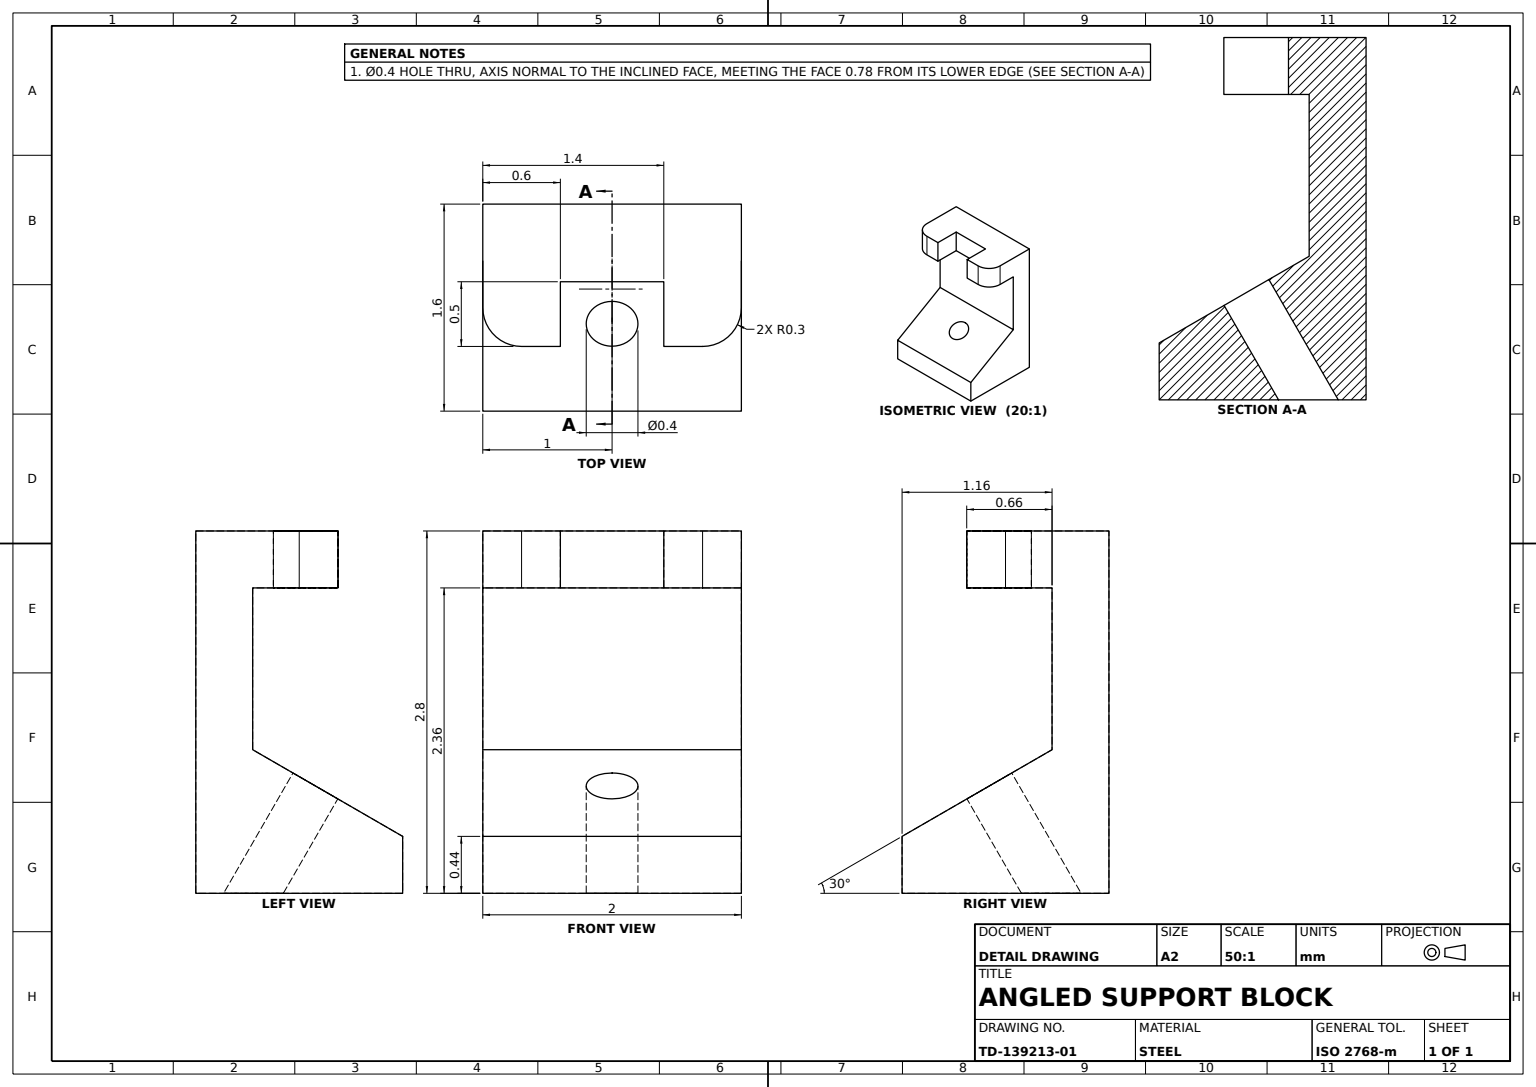
SolidWorks part; units mm, degrees
material "Plain Carbon Steel"
ref_plane "Front Plane" through (0, 0, 0) normal (0, 0, 1) x (1, 0, 0)
ref_plane "Top Plane" through (0, 0, 0) normal (0, 1, 0) x (1, 0, 0)
ref_plane "Right Plane" through (0, 0, 0) normal (1, 0, 0) x (0, 0, -1)
sketch "L Profile Sketch" plane through (0, 0, 0) normal (1, 0, 0) x (0, 0, -1)
  line L0 (0, 0) -> (1.6, 0)
  line L1 (1.6, 0) -> (1.6, 2.8)
  line L2 (1.6, 2.8) -> (0.5, 2.8)
  line L3 (0.5, 2.8) -> (0.5, 2.36)
  line L4 (0.5, 2.36) -> (1.16, 2.36)
  line L7 (0, 0) -> (0, 0.44)
  line L8 (0, 0.44) -> (1.16, 1.1097)
  line L9 (1.16, 2.36) -> (1.16, 1.1097)
  dimension "D1" = 1.16
  dimension "D2" = 1.6
  dimension "D3" = 30
  dimension "D4" = 0.66
  dimension "D5" = 0.44
  dimension "D6" = 2.36
  dimension "D7" = 0.44
extrude "L Bracket Body 2mm" add sketch "L Profile Sketch" along normal mid plane 2
sketch "Upright Slot Sketch" plane through (0, 2.8, 0) normal (0, 1, 0) x (1, 0, 0)
  line L0 (-1, 1.6) -> (-1, 0.5) construction
  line L3 (0.4, 1) -> (-0.4, 1)
  line L4 (-0.4, 1) -> (-0.4, 0.5)
  line L5 (1, 0.5) -> (-1, 0.5) construction
  line L10 (0.4, 1) -> (0.4, 0.5)
  line L11 (0.4, 0.5) -> (-0.4, 0.5)
  dimension "D1" = 0.6
  dimension "D2" = 1.4
  dimension "D3" = 0.5
extrude "Upright Slot Cut 1mm Deep" cut sketch "Upright Slot Sketch" against normal blind 1
fillet "Corner Fillet R0.3 A" radius 0.3 1 edges at (1, 2.58, -0.5)
fillet "Corner Fillet R0.3 B" radius 0.3 1 edges at (-1, 2.58, -0.5)
sketch "Angled Face Hole Sketch" plane through (0, 0.33, 0.1905) normal (0, 0.866, 0.5) x (1, 0, 0)
  line L0 (-1, 1.5595) -> (-1, 0.22) construction
  line L1 (1, 0.22) -> (-1, 0.22) construction
  circle A0 centre (0, 0.9995) radius 0.2
  dimension "D1" = 0.4
  dimension "D2" = 1
  dimension "D3" = 0.7795
extrude "Angled Face Hole Cut" cut sketch "Angled Face Hole Sketch" against normal blind 2
